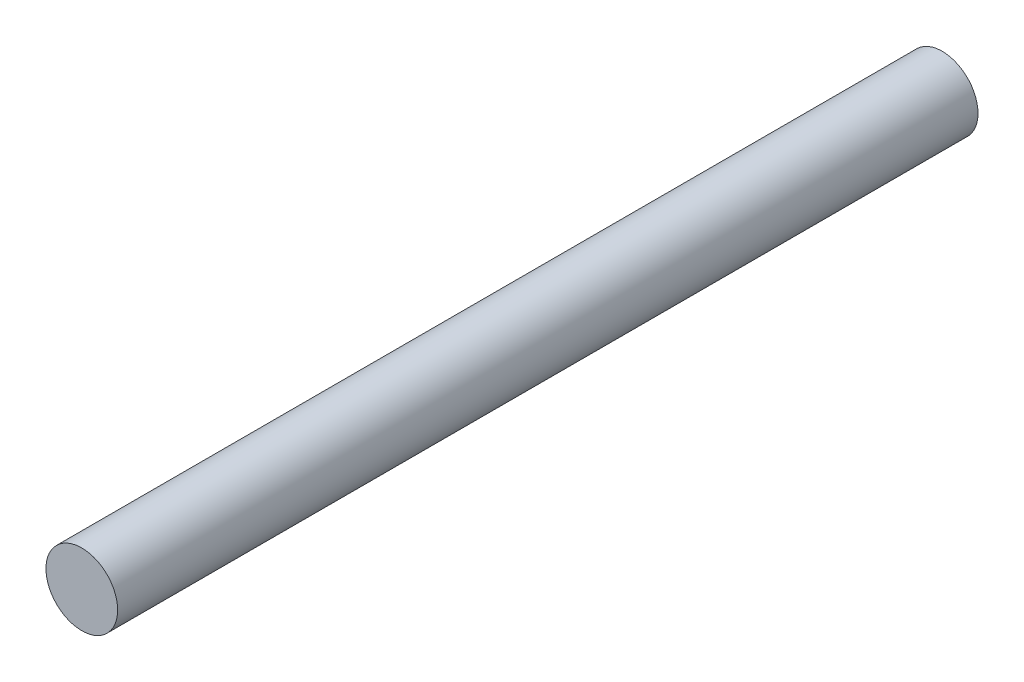
ISO-10303-21;
HEADER;
FILE_DESCRIPTION(('STEP AP214'),'2;1');
FILE_NAME('part.step','',(''),(''),'','','');
FILE_SCHEMA(('AUTOMOTIVE_DESIGN { 1 0 10303 214 1 1 1 1 }'));
ENDSEC;
DATA;
#1=APPLICATION_CONTEXT('core data for automotive mechanical design processes');
#2=APPLICATION_PROTOCOL_DEFINITION('international standard','automotive_design',2000,#1);
#3=PRODUCT_CONTEXT('',#1,'mechanical');
#4=PRODUCT('Part','Part','',(#3));
#5=PRODUCT_RELATED_PRODUCT_CATEGORY('part','',(#4));
#6=PRODUCT_DEFINITION_FORMATION('','',#4);
#7=PRODUCT_DEFINITION_CONTEXT('part definition',#1,'design');
#8=PRODUCT_DEFINITION('design','',#6,#7);
#9=PRODUCT_DEFINITION_SHAPE('','',#8);
#10=(LENGTH_UNIT() NAMED_UNIT(*) SI_UNIT(.MILLI.,.METRE.));
#11=(NAMED_UNIT(*) PLANE_ANGLE_UNIT() SI_UNIT($,.RADIAN.));
#12=(NAMED_UNIT(*) SI_UNIT($,.STERADIAN.) SOLID_ANGLE_UNIT());
#13=UNCERTAINTY_MEASURE_WITH_UNIT(LENGTH_MEASURE(1.E-05),#10,'distance_accuracy_value','');
#14=(GEOMETRIC_REPRESENTATION_CONTEXT(3) GLOBAL_UNCERTAINTY_ASSIGNED_CONTEXT((#13)) GLOBAL_UNIT_ASSIGNED_CONTEXT((#10,
#11,#12)) REPRESENTATION_CONTEXT('',''));
#15=CARTESIAN_POINT('',(0.,0.,0.));
#16=DIRECTION('',(0.,0.,1.));
#17=DIRECTION('',(1.,0.,0.));
#18=AXIS2_PLACEMENT_3D('',#15,#16,#17);
#19=CARTESIAN_POINT('',(0.,0.,36.));
#20=DIRECTION('',(0.,0.,-1.));
#21=DIRECTION('',(-1.,0.,0.));
#22=AXIS2_PLACEMENT_3D('',#19,#20,#21);
#23=CYLINDRICAL_SURFACE('',#22,3.);
#24=CARTESIAN_POINT('',(0.,0.,36.));
#25=DIRECTION('',(0.,0.,1.));
#26=DIRECTION('',(1.,0.,0.));
#27=AXIS2_PLACEMENT_3D('',#24,#25,#26);
#28=CIRCLE('',#27,3.);
#29=CARTESIAN_POINT('',(3.,0.,36.));
#30=VERTEX_POINT('',#29);
#31=EDGE_CURVE('E10',#30,#30,#28,.T.);
#32=ORIENTED_EDGE('',*,*,#31,.F.);
#33=EDGE_LOOP('',(#32));
#34=FACE_BOUND('',#33,.T.);
#35=CARTESIAN_POINT('',(0.,0.,-36.));
#36=DIRECTION('',(0.,0.,1.));
#37=DIRECTION('',(1.,0.,0.));
#38=AXIS2_PLACEMENT_3D('',#35,#36,#37);
#39=CIRCLE('',#38,3.);
#40=CARTESIAN_POINT('',(3.,0.,-36.));
#41=VERTEX_POINT('',#40);
#42=EDGE_CURVE('E37',#41,#41,#39,.T.);
#43=ORIENTED_EDGE('',*,*,#42,.T.);
#44=EDGE_LOOP('',(#43));
#45=FACE_BOUND('',#44,.T.);
#46=ADVANCED_FACE('F40',(#34,#45),#23,.T.);
#47=CARTESIAN_POINT('',(0.,0.,36.));
#48=DIRECTION('',(0.,0.,1.));
#49=DIRECTION('',(1.,0.,0.));
#50=AXIS2_PLACEMENT_3D('',#47,#48,#49);
#51=PLANE('',#50);
#52=ORIENTED_EDGE('',*,*,#31,.T.);
#53=EDGE_LOOP('',(#52));
#54=FACE_BOUND('',#53,.T.);
#55=ADVANCED_FACE('F55',(#54),#51,.T.);
#56=CARTESIAN_POINT('',(0.,0.,-36.));
#57=DIRECTION('',(0.,0.,1.));
#58=DIRECTION('',(1.,0.,0.));
#59=AXIS2_PLACEMENT_3D('',#56,#57,#58);
#60=PLANE('',#59);
#61=ORIENTED_EDGE('',*,*,#42,.F.);
#62=EDGE_LOOP('',(#61));
#63=FACE_BOUND('',#62,.T.);
#64=ADVANCED_FACE('F49',(#63),#60,.F.);
#65=CLOSED_SHELL('',(#46,#55,#64));
#66=MANIFOLD_SOLID_BREP('B2',#65);
#67=ADVANCED_BREP_SHAPE_REPRESENTATION('',(#18,#66),#14);
#68=SHAPE_DEFINITION_REPRESENTATION(#9,#67);
ENDSEC;
END-ISO-10303-21;
